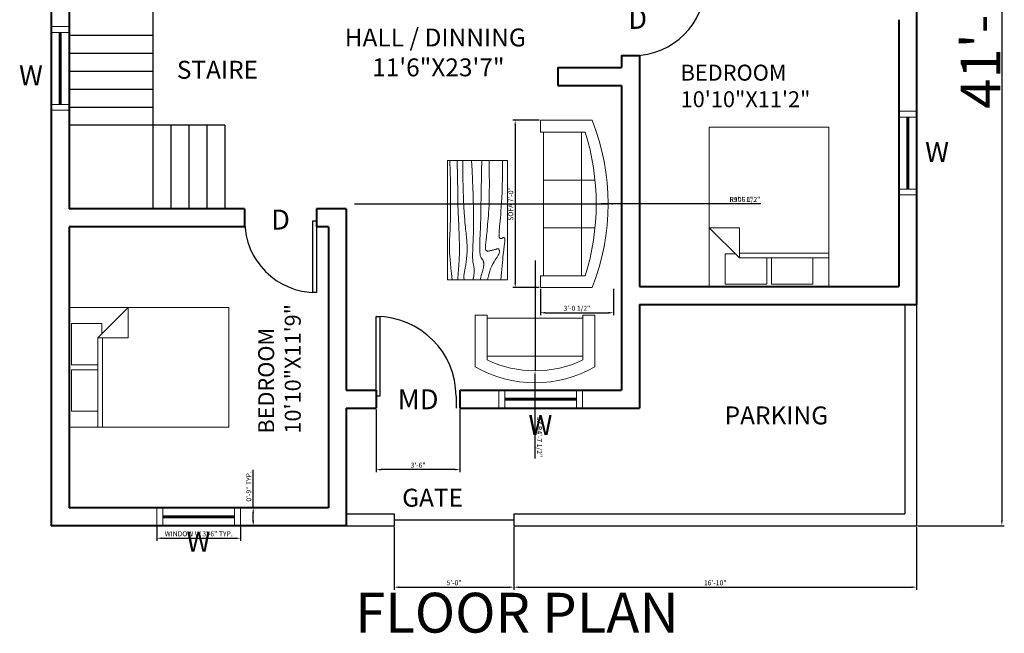
# Model space of a CAD drawing. Units: inches. Extents: x 4878 to 9282, y 5367 to 6617.
# Tile 10 of 14: x 8028 to 8522, y 6010 to 6318. Entities that reach past the tile are written whole.
import ezdxf

# ---------------------------------------------------------------- set-up
doc = ezdxf.new("R2010")
doc.units = ezdxf.units.IN
for name, color, linetype, lineweight in [('A-ANNO-DIMS', 2, 'Continuous', 18), ('A-ANNO-TEXT', 7, 'Continuous', 18), ('A-ANNO-TITL', 3, 'Continuous', 30), ('A-AREA-IDEN', 4, 'Continuous', 18), ('A-DOOR', 3, 'Continuous', 25), ('A-FLOR-STRS', 7, 'Continuous', 25), ('A-FURN', 8, 'Continuous', 18), ('A-GLAZ', 30, 'Continuous', 20), ('A-SITE', 7, 'Continuous', 25), ('A-WALL', 7, 'Continuous', 40)]:
    doc.layers.add(name, color=color, linetype=linetype, lineweight=lineweight)
doc.styles.get("Standard").update_dxf_attribs({"font": 'arial.ttf'})
doc.dimstyles.new('ISO-25', dxfattribs={"dimtxt": 2.5, "dimasz": 2.5, "dimexe": 1.25, "dimexo": 0.625, "dimtad": 1, "dimdec": 0, "dimlunit": 3, "dimtxsty": 'Standard', "dimcen": 2.5, "dimadec": 0, "dimazin": 0, "dimtfac": 1, "dimtdec": 0, "dimtmove": 0, "dimatfit": 3, "dimfxl": 1, "dimarcsym": 0})

# ---------------------------------------------------------------- blocks, each defined once
blk = doc.blocks.new('Bed - Queen')
for p, q in [((0, -80.00003), (0, 0)), ((0, 0), (59.99999, 0)), ((59.99999, 0), (59.99999, -80.00003)), ((7.99999, -1.2), (28.79998, -1.2)), ((7.99999, -14.4), (7.99999, -1.2)), ((28.79998, -1.2), (28.79998, -14.4)), ((31.19999, -1.2), (51.99999, -1.2)), ((31.19999, -14.4), (31.19999, -1.2)), ((51.99999, -1.2), (51.99999, -16.4)), ((0, -14.4), (44.8, -14.4)), ((59.99999, -29.6), (44.8, -14.4)), ((44.8, -14.4), (44.8, -29.6)), ((44.8, -16.8), (0, -16.8)), ((51.99999, -16.4), (46.79936, -16.4)), ((44.8, -29.6), (59.99999, -29.6)), ((59.99999, -80.00003), (0, -80.00003))]:
    blk.add_line(p, q)
blk = doc.blocks.new('Sofa - Roundback 7 ft.')
for p, q in [((-12.00002, -32.4421), (-12.00003, -6.5971)), ((11.99997, -32.4421), (11.99998, -6.5971)), ((-36.000027, -34), (-36.000027, -11.4696)), ((-35.999844, -13.3819), (35.9998, -13.3819)), ((35.99998, -34), (35.99998, -11.4696)), ((-36.000027, -32.4421), (35.99998, -32.4421))]:
    blk.add_line(p, q)
for points in [[(-36.000027, -34), (-42.000027, -34), (-42.000027, -8)], [(41.99998, -8), (41.99998, -34), (35.99998, -34)]]:
    blk.add_lwpolyline(points)
for centre, radius, start, end in [((0, -114.25), 114.25, 68.43141, 111.5686), ((-0.00001, -127.1968), 121.1968, 72.72033, 107.2797)]:
    blk.add_arc(centre, radius, start, end)
blk = doc.blocks.new('Sofa - Roundback Loveseat 5 ft.')
for p, q in [((0, -32.44198), (0, -5.99998)), ((-24, -33.99998), (-24, -11.46958)), ((-23.9998, -13.38178), (23.99986, -13.38178)), ((24.00004, -33.99998), (24.00004, -11.46958)), ((-24, -32.44198), (24.00004, -32.44198))]:
    blk.add_line(p, q)
for points in [[(-24, -33.99998), (-30, -33.99998), (-30, -7.99998)], [(30.00004, -7.99998), (30.00004, -33.99998), (24.00004, -33.99998)]]:
    blk.add_lwpolyline(points)
for centre, radius, start, end in [((0, -60.24998), 60.24998, 60.13715, 119.8628), ((0, -61.38438), 55.38444, 64.32083, 115.6792)]:
    blk.add_arc(centre, radius, start, end)
blk = doc.blocks.new('Table - Rectangular Woodgrain 60 x 30 in.')
for p, q in [((0, 0), (0, -30)), ((60, 0), (0, 0)), ((60, -30), (60, 0)), ((0, -30), (60, -30))]:
    blk.add_line(p, q)
for points in [[(0, -2.4), (4.8155, -2.418), (9.0302, -2.4688), (12.709, -2.5477), (15.9167, -2.65), (18.7181, -2.7711), (21.1781, -2.9063), (23.3616, -3.0508), (25.3333, -3.2), (27.1477, -3.3495), (28.8172, -3.4958), (30.3437, -3.636), (31.7291, -3.7667), (32.9756, -3.8849), (34.0849, -3.9875), (35.059, -4.0714), (35.9, -4.1334), (36.6114, -4.1711), (37.2041, -4.1854), (37.6906, -4.1779), (38.0833, -4.15), (38.3948, -4.1034), (38.6375, -4.0396), (38.8239, -3.9602), (38.9666, -3.8667), (39.0764, -3.7608), (39.1573, -3.6448), (39.2116, -3.521), (39.2416, -3.3917), (39.2498, -3.2593), (39.2385, -3.1261), (39.21, -2.9944), (39.1666, -2.8667), (39.111, -2.7447), (39.0468, -2.6281), (38.978, -2.5163), (38.9083, -2.4083), (38.8418, -2.3035), (38.7823, -2.201), (38.7337, -2.1001), (38.7, -2), (38.6844, -1.9003), (38.6875, -1.8021), (38.7094, -1.707), (38.75, -1.6167), (38.8094, -1.5326), (38.8875, -1.4563), (38.9844, -1.3893), (39.1, -1.3333), (39.2351, -1.2896), (39.3937, -1.2583), (39.5804, -1.2396), (39.8, -1.2333), (40.057, -1.2396), (40.3562, -1.2583), (40.7023, -1.2896), (41.1, -1.3333), (41.5547, -1.3895), (42.0755, -1.4573), (42.6721, -1.5361), (43.3542, -1.625), (44.1316, -1.7233), (45.014, -1.8302), (46.0114, -1.9449), (47.1333, -2.0667), (48.3862, -2.1947), (49.7625, -2.3281), (51.2513, -2.4663), (52.8416, -2.6083), (54.5226, -2.7535), (56.2833, -2.9011), (58.1127, -3.0501), (60, -3.2)], [(0, -9.2), (6.5759, -9.0858), (11.9385, -9.0365), (16.2527, -9.0418), (19.6833, -9.0917), (22.3952, -9.1759), (24.5531, -9.2844), (26.322, -9.4069), (27.8666, -9.5333), (29.3241, -9.6553), (30.7203, -9.7719), (32.0532, -9.8837), (33.3208, -9.9917), (34.5213, -10.0965), (35.6526, -10.199), (36.7128, -10.2999), (37.7, -10.4), (38.6129, -10.4996), (39.4531, -10.5969), (40.223, -10.6895), (40.925, -10.775), (41.5613, -10.8512), (42.1344, -10.9156), (42.6465, -10.966), (43.1, -11), (43.4976, -11.0158), (43.8437, -11.0136), (44.143, -10.9942), (44.4, -10.9583), (44.6195, -10.9069), (44.8062, -10.8406), (44.9648, -10.7603), (45.1, -10.6667), (45.2155, -10.5598), (45.3114, -10.4365), (45.3871, -10.2929), (45.4416, -10.125), (45.4743, -9.929), (45.4844, -9.7011), (45.4709, -9.4371), (45.4333, -9.1333), (45.3716, -8.7883), (45.2896, -8.4104), (45.1919, -8.0107), (45.0833, -7.6), (44.9685, -7.1893), (44.8521, -6.7896), (44.7388, -6.4117), (44.6333, -6.0667), (44.54, -5.7628), (44.4614, -5.4979), (44.4001, -5.2675), (44.3583, -5.0667), (44.3384, -4.8909), (44.3427, -4.7354), (44.3736, -4.5956), (44.4333, -4.4667), (44.5236, -4.3453), (44.6427, -4.2333), (44.7884, -4.1339), (44.9583, -4.05), (45.1501, -3.9849), (45.3614, -3.9417), (45.59, -3.9234), (45.8333, -3.9333), (46.0915, -3.9749), (46.3734, -4.0531), (46.6906, -4.1736), (47.0542, -4.3417), (47.4756, -4.5629), (47.9661, -4.8427), (48.5372, -5.1866), (49.2, -5.6), (49.9676, -6.0844), (50.8594, -6.625), (51.8965, -7.2031), (53.1, -7.8), (54.491, -8.3969), (56.0906, -8.975), (57.9199, -9.5156), (60, -10)], [(0, -12.8), (5.1847, -12.9322), (9.6213, -13.0323), (13.3963, -13.1059), (16.5958, -13.1583), (19.3063, -13.1952), (21.614, -13.2219), (23.6054, -13.2439), (25.3666, -13.2667), (26.9728, -13.2947), (28.4531, -13.3281), (29.8256, -13.3663), (31.1083, -13.4083), (32.3191, -13.4535), (33.476, -13.501), (34.597, -13.5501), (35.7, -13.6), (36.7984, -13.6497), (37.8875, -13.6979), (38.9578, -13.743), (40, -13.7833), (41.0047, -13.8174), (41.9625, -13.8438), (42.864, -13.8607), (43.7, -13.8667), (44.4631, -13.8604), (45.1552, -13.8417), (45.7801, -13.8104), (46.3416, -13.7667), (46.8439, -13.7104), (47.2906, -13.6417), (47.6858, -13.5604), (48.0333, -13.4667), (48.3375, -13.3608), (48.6042, -13.2448), (48.8396, -13.121), (49.05, -12.9917), (49.2417, -12.8593), (49.4208, -12.7261), (49.5937, -12.5944), (49.7667, -12.4667), (49.9452, -12.3451), (50.1323, -12.2313), (50.3303, -12.1268), (50.5416, -12.0333), (50.7686, -11.9524), (51.0135, -11.8854), (51.2788, -11.8341), (51.5666, -11.8), (51.8785, -11.7843), (52.2116, -11.7865), (52.562, -11.8059), (52.926, -11.8417), (53.2998, -11.8931), (53.6795, -11.9594), (54.0614, -12.0397), (54.4416, -12.1333), (54.8223, -12.2401), (55.2293, -12.3625), (55.6942, -12.5037), (56.2489, -12.6667), (56.9251, -12.8547), (57.7545, -13.0708), (58.7689, -13.3182), (60, -13.6)], [(0, -18), (5.124, -17.7273), (9.6609, -17.5057), (13.6705, -17.3303), (17.2125, -17.1958), (20.3467, -17.0973), (23.1328, -17.0297), (25.6307, -16.9878), (27.9, -16.9667), (29.9928, -16.9617), (31.9302, -16.9703), (33.7254, -16.9907), (35.3917, -17.0208), (36.9423, -17.0588), (38.3906, -17.1026), (39.7499, -17.1503), (41.0333, -17.2), (42.2519, -17.2496), (43.4073, -17.2969), (44.4986, -17.3395), (45.525, -17.375), (46.4858, -17.4012), (47.3802, -17.4156), (48.2074, -17.416), (48.9667, -17.4), (49.6583, -17.3662), (50.2872, -17.3167), (50.8595, -17.2547), (51.3812, -17.1833), (51.8584, -17.1057), (52.2971, -17.025), (52.7034, -16.9443), (53.0833, -16.8667), (53.443, -16.7951), (53.789, -16.7313), (54.128, -16.6768), (54.4666, -16.6334), (54.8115, -16.6024), (55.1693, -16.5854), (55.5465, -16.5841), (55.95, -16.6), (56.3828, -16.6337), (56.8346, -16.6823), (57.2915, -16.7418), (57.7396, -16.8084), (58.165, -16.878), (58.5539, -16.9469), (58.8924, -17.0111), (59.1666, -17.0667), (59.3679, -17.1107), (59.5078, -17.1438), (59.6032, -17.1675), (59.6708, -17.1833), (59.7275, -17.193), (59.7901, -17.1979), (59.8753, -17.1998), (60, -17.2)], [(0, -22.4), (8.0098, -22.2501), (14.4094, -22.1011), (19.4168, -21.9535), (23.25, -21.8083), (26.1269, -21.6663), (28.2656, -21.5281), (29.884, -21.3947), (31.2, -21.2667), (32.3967, -21.1448), (33.5172, -21.0292), (34.5697, -20.9198), (35.5625, -20.8167), (36.5037, -20.7198), (37.4015, -20.6292), (38.2642, -20.5448), (39.1, -20.4667), (39.9164, -20.3951), (40.7187, -20.3313), (41.5117, -20.2768), (42.3, -20.2333), (43.0883, -20.2024), (43.8812, -20.1854), (44.6836, -20.1841), (45.5, -20.2), (46.3328, -20.234), (47.1747, -20.2844), (48.0163, -20.3488), (48.8479, -20.425), (49.66, -20.5106), (50.4429, -20.6031), (51.1872, -20.7004), (51.8833, -20.8), (52.5246, -20.8999), (53.1166, -20.9995), (53.6681, -21.0983), (54.1875, -21.1958), (54.6834, -21.2919), (55.1646, -21.3859), (55.6394, -21.4777), (56.1167, -21.5667), (56.6028, -21.6515), (57.0961, -21.7266), (57.5929, -21.7852), (58.0896, -21.8208), (58.5823, -21.8268), (59.0674, -21.7964), (59.5412, -21.723), (60, -21.6)], [(0, -25.2), (8.6355, -25.0504), (15.7026, -24.9031), (21.4049, -24.7606), (25.9458, -24.625), (29.529, -24.4988), (32.3578, -24.3844), (34.6359, -24.284), (36.5667, -24.2), (38.3213, -24.1341), (39.9417, -24.0854), (41.437, -24.0523), (42.8167, -24.0333), (44.0901, -24.0268), (45.2667, -24.0313), (46.3557, -24.0451), (47.3667, -24.0667), (48.309, -24.0947), (49.1928, -24.1287), (50.0284, -24.168), (50.826, -24.2125), (51.5959, -24.2617), (52.3483, -24.3151), (53.0935, -24.3725), (53.8417, -24.4334), (54.6009, -24.497), (55.3699, -24.561), (56.1454, -24.6226), (56.9239, -24.6792), (57.7021, -24.7279), (58.4764, -24.7662), (59.2435, -24.7911), (60, -24.8)], [(0, -28.8), (5.6867, -28.6681), (10.45, -28.5698), (14.407, -28.5012), (17.675, -28.4584), (20.3711, -28.4374), (22.6125, -28.4344), (24.5164, -28.4455), (26.2, -28.4667), (27.762, -28.4947), (29.2276, -28.5281), (30.6033, -28.5663), (31.8958, -28.6084), (33.1118, -28.6535), (34.2578, -28.7011), (35.3405, -28.7501), (36.3666, -28.8), (37.3443, -28.8497), (38.288, -28.8974), (39.2137, -28.9412), (40.1375, -28.9792), (41.0753, -29.0093), (42.0432, -29.0297), (43.0572, -29.0384), (44.1333, -29.0333), (45.2936, -29.0114), (46.5843, -28.9641), (48.0579, -28.8816), (49.7666, -28.7542), (51.7629, -28.5721), (54.0989, -28.3255), (56.8272, -28.0048), (60, -27.6)]]:
    blk.add_lwpolyline(points)
blk = doc.blocks.new('*U18')
for p, q in [((0, 0), (0, -6)), ((40, 0), (40, -6))]:
    blk.add_line(p, q)
blk.add_lwpolyline([(0, 0), (0, 40), (1.75, 40), (1.75, 0)], close=True)
blk.add_arc((0, 0), 40, 0, 90)
blk = doc.blocks.new('*U20')
for p, q in [((-36, 0), (-36, 6)), ((0, 0), (0, 6))]:
    blk.add_line(p, q)
blk.add_lwpolyline([(0, 0), (0, -36), (-1.75, -36), (-1.75, 0)], close=True)
blk.add_arc((0, 0), 36, 180, 270)
blk = doc.blocks.new('*D26')
at = {"layer": 'A-ANNO-DIMS', "color": 0, "lineweight": -2, "transparency": 16777216}
for p, q in [((8478.72, 6557.77), (8522.05, 6557.77)), ((8520.8, 6555.27), (8520.8, 6066.27)), ((8478.72, 6063.77), (8522.05, 6063.77))]:
    blk.add_line(p, q, dxfattribs=at)
at = {"layer": 'A-ANNO-DIMS', "color": 0, "transparency": 16777216}
for points in [[(8520.39, 6555.27), (8521.22, 6555.27), (8520.8, 6557.77)], [(8520.39, 6066.27), (8521.22, 6066.27), (8520.8, 6063.77)]]:
    blk.add_solid(points, dxfattribs=at)
at = {"layer": 'Defpoints', "color": 0, "transparency": 16777216}
for p in [(8478.1, 6557.77), (8478.1, 6063.77), (8520.8, 6063.77)]:
    blk.add_point(p, dxfattribs=at)
at = {"layer": 'A-ANNO-DIMS', "color": 0, "transparency": 16777216, "insert": (8510.14, 6310.77), "char_height": 2.5, "attachment_point": 5, "rotation": 90}
blk.add_mtext('{\\H8x;41\'-2"}', dxfattribs=at)
blk = doc.blocks.new('WINDOW-PLAN-36IN')
for p, q in [((0, 0), (0, 9)), ((3, 0), (3, 9)), ((3, 5), (39, 5)), ((39, 0), (39, 9)), ((42, 0), (42, 9)), ((3, 4.5), (39, 4.5)), ((3, 4), (39, 4))]:
    blk.add_line(p, q)
blk = doc.blocks.new('*D39')
at = {"layer": 'A-ANNO-DIMS', "color": 0, "lineweight": -2, "transparency": 16777216}
for p, q in [((8097.1, 6063.15), (8097.1, 6056.22)), ((8139.1, 6063.15), (8139.1, 6056.22)), ((8099.6, 6057.47), (8136.6, 6057.47))]:
    blk.add_line(p, q, dxfattribs=at)
at = {"layer": 'A-ANNO-DIMS', "color": 0, "transparency": 16777216}
for points in [[(8099.6, 6057.89), (8099.6, 6057.05), (8097.1, 6057.47)], [(8136.6, 6057.89), (8136.6, 6057.05), (8139.1, 6057.47)]]:
    blk.add_solid(points, dxfattribs=at)
at = {"layer": 'Defpoints', "color": 0, "transparency": 16777216}
for p in [(8097.1, 6063.77), (8139.1, 6063.77), (8139.1, 6057.47)]:
    blk.add_point(p, dxfattribs=at)
at = {"layer": 'A-ANNO-DIMS', "color": 0, "transparency": 16777216, "insert": (8118.1, 6059.39), "char_height": 2.5, "attachment_point": 5}
blk.add_mtext('WINDOW W 3\'-6" TYP.', dxfattribs=at)
blk = doc.blocks.new('*D40')
at = {"layer": 'A-ANNO-DIMS', "color": 0, "lineweight": -2, "transparency": 16777216}
for p, q in [((8145.4, 6072.77), (8145.4, 6091.76)), ((8139.72, 6072.77), (8146.65, 6072.77)), ((8145.4, 6066.27), (8145.4, 6070.27)), ((8139.72, 6063.77), (8146.65, 6063.77))]:
    blk.add_line(p, q, dxfattribs=at)
at = {"layer": 'A-ANNO-DIMS', "color": 0, "transparency": 16777216}
for points in [[(8144.98, 6070.27), (8145.81, 6070.27), (8145.4, 6072.77)], [(8144.98, 6066.27), (8145.81, 6066.27), (8145.4, 6063.77)]]:
    blk.add_solid(points, dxfattribs=at)
at = {"layer": 'Defpoints', "color": 0, "transparency": 16777216}
for p in [(8139.1, 6072.77), (8145.4, 6072.77), (8139.1, 6063.77)]:
    blk.add_point(p, dxfattribs=at)
at = {"layer": 'A-ANNO-DIMS', "color": 0, "transparency": 16777216, "insert": (8143.49, 6083.52), "char_height": 2.5, "attachment_point": 5, "rotation": 90}
blk.add_mtext('0\'-9" TYP.', dxfattribs=at)
blk = doc.blocks.new('*D63')
at = {"layer": 'A-ANNO-DIMS', "color": 0, "lineweight": -2, "transparency": 16777216}
for p, q in [((8288.76, 6267.27), (8275.54, 6267.27)), ((8276.79, 6264.77), (8276.79, 6185.77)), ((8288.76, 6183.27), (8275.54, 6183.27))]:
    blk.add_line(p, q, dxfattribs=at)
at = {"layer": 'A-ANNO-DIMS', "color": 0, "transparency": 16777216}
for points in [[(8276.37, 6264.77), (8277.21, 6264.77), (8276.79, 6267.27)], [(8276.37, 6185.77), (8277.21, 6185.77), (8276.79, 6183.27)]]:
    blk.add_solid(points, dxfattribs=at)
at = {"layer": 'Defpoints', "color": 0, "transparency": 16777216}
for p in [(8289.39, 6267.27), (8276.79, 6183.27), (8289.39, 6183.27)]:
    blk.add_point(p, dxfattribs=at)
at = {"layer": 'A-ANNO-DIMS', "color": 0, "transparency": 16777216, "insert": (8274.87, 6225.27), "char_height": 2.5, "attachment_point": 5, "rotation": 90}
blk.add_mtext('SOFA 7\'-0"', dxfattribs=at)
blk = doc.blocks.new('*D64')
at = {"layer": 'A-ANNO-DIMS', "color": 0, "lineweight": -2, "transparency": 16777216}
for p, q in [((8289.39, 6182.64), (8289.39, 6169.42)), ((8326.06, 6182.64), (8326.06, 6169.42)), ((8291.89, 6170.67), (8323.56, 6170.67))]:
    blk.add_line(p, q, dxfattribs=at)
at = {"layer": 'A-ANNO-DIMS', "color": 0, "transparency": 16777216}
for points in [[(8291.89, 6171.08), (8291.89, 6170.25), (8289.39, 6170.67)], [(8323.56, 6171.08), (8323.56, 6170.25), (8326.06, 6170.67)]]:
    blk.add_solid(points, dxfattribs=at)
at = {"layer": 'Defpoints', "color": 0, "transparency": 16777216}
for p in [(8289.39, 6183.27), (8326.06, 6183.27), (8326.06, 6170.67)]:
    blk.add_point(p, dxfattribs=at)
at = {"layer": 'A-ANNO-DIMS', "color": 0, "transparency": 16777216, "insert": (8307.72, 6172.58), "char_height": 2.5, "attachment_point": 5}
blk.add_mtext('3\'-0 1/2"', dxfattribs=at)
blk = doc.blocks.new('*D109')
at = {"layer": 'A-ANNO-DIMS', "color": 0, "lineweight": -2, "transparency": 16777216}
for p, q in [((8207.1, 6122.15), (8207.1, 6090.67)), ((8249.1, 6122.15), (8249.1, 6090.67)), ((8246.6, 6091.92), (8209.6, 6091.92))]:
    blk.add_line(p, q, dxfattribs=at)
at = {"layer": 'A-ANNO-DIMS', "color": 0, "transparency": 16777216}
for points in [[(8209.6, 6092.34), (8209.6, 6091.5), (8207.1, 6091.92)], [(8246.6, 6092.34), (8246.6, 6091.5), (8249.1, 6091.92)]]:
    blk.add_solid(points, dxfattribs=at)
at = {"layer": 'Defpoints', "color": 0, "transparency": 16777216}
for p in [(8207.1, 6122.77), (8249.1, 6122.77), (8207.1, 6091.92)]:
    blk.add_point(p, dxfattribs=at)
at = {"layer": 'A-ANNO-DIMS', "color": 0, "transparency": 16777216, "insert": (8228.1, 6093.82), "char_height": 2.5, "attachment_point": 5}
blk.add_mtext('3\'-6"', dxfattribs=at)
blk = doc.blocks.new('*D111')
at = {"layer": 'A-ANNO-DIMS', "color": 0, "lineweight": -2, "transparency": 16777216}
for p, q in [((8216.1, 6063.15), (8216.1, 6031.67)), ((8276.1, 6063.15), (8276.1, 6031.67)), ((8218.6, 6032.92), (8273.6, 6032.92))]:
    blk.add_line(p, q, dxfattribs=at)
at = {"layer": 'A-ANNO-DIMS', "color": 0, "transparency": 16777216}
for points in [[(8218.6, 6033.34), (8218.6, 6032.5), (8216.1, 6032.92)], [(8273.6, 6033.34), (8273.6, 6032.5), (8276.1, 6032.92)]]:
    blk.add_solid(points, dxfattribs=at)
at = {"layer": 'Defpoints', "color": 0, "transparency": 16777216}
for p in [(8216.1, 6063.77), (8276.1, 6063.77), (8276.1, 6032.92)]:
    blk.add_point(p, dxfattribs=at)
at = {"layer": 'A-ANNO-DIMS', "color": 0, "transparency": 16777216, "insert": (8246.1, 6034.82), "char_height": 2.5, "attachment_point": 5}
blk.add_mtext('5\'-0"', dxfattribs=at)
blk = doc.blocks.new('*D112')
at = {"layer": 'A-ANNO-DIMS', "color": 0, "lineweight": -2, "transparency": 16777216}
for p, q in [((8276.1, 6063.15), (8276.1, 6031.67)), ((8478.1, 6063.15), (8478.1, 6031.67)), ((8278.6, 6032.92), (8475.6, 6032.92))]:
    blk.add_line(p, q, dxfattribs=at)
at = {"layer": 'A-ANNO-DIMS', "color": 0, "transparency": 16777216}
for points in [[(8278.6, 6033.34), (8278.6, 6032.5), (8276.1, 6032.92)], [(8475.6, 6033.34), (8475.6, 6032.5), (8478.1, 6032.92)]]:
    blk.add_solid(points, dxfattribs=at)
at = {"layer": 'Defpoints', "color": 0, "transparency": 16777216}
for p in [(8276.1, 6063.77), (8478.1, 6063.77), (8478.1, 6032.92)]:
    blk.add_point(p, dxfattribs=at)
at = {"layer": 'A-ANNO-DIMS', "color": 0, "transparency": 16777216, "insert": (8377.1, 6034.82), "char_height": 2.5, "attachment_point": 5}
blk.add_mtext('16\'-10"', dxfattribs=at)
blk = doc.blocks.new('*D123')
at = {"layer": 'A-ANNO-DIMS', "color": 0, "lineweight": -2, "transparency": 16777216}
for p, q in [((8286.73, 6196.91), (8286.73, 6141.53)), ((8286.73, 6097.55), (8286.73, 6139.03))]:
    blk.add_line(p, q, dxfattribs=at)
at = {"layer": 'A-ANNO-DIMS', "color": 0, "transparency": 16777216}
blk.add_solid([(8287.15, 6139.03), (8286.32, 6139.03), (8286.73, 6141.53)], dxfattribs=at)
at = {"layer": 'Defpoints', "color": 0, "transparency": 16777216}
for p in [(8286.73, 6196.91), (8286.73, 6141.53)]:
    blk.add_point(p, dxfattribs=at)
at = {"layer": 'A-ANNO-DIMS', "color": 0, "transparency": 16777216, "insert": (8288.65, 6108.29), "char_height": 2.5, "attachment_point": 5, "rotation": 270.0004}
blk.add_mtext('3X R4\'-7 1/2"', dxfattribs=at)
blk = doc.blocks.new('*D124')
at = {"layer": 'A-ANNO-DIMS', "color": 0, "lineweight": -2, "transparency": 16777216}
for p, q in [((8196.19, 6225.27), (8317.39, 6225.27)), ((8396.22, 6225.27), (8319.89, 6225.27))]:
    blk.add_line(p, q, dxfattribs=at)
at = {"layer": 'A-ANNO-DIMS', "color": 0, "transparency": 16777216}
blk.add_solid([(8319.89, 6225.68), (8319.89, 6224.85), (8317.39, 6225.27)], dxfattribs=at)
at = {"layer": 'Defpoints', "color": 0, "transparency": 16777216}
for p in [(8196.19, 6225.27), (8317.39, 6225.27)]:
    blk.add_point(p, dxfattribs=at)
at = {"layer": 'A-ANNO-DIMS', "color": 0, "transparency": 16777216, "insert": (8390.11, 6227.17), "char_height": 2.5, "attachment_point": 5, "rotation": 360}
blk.add_mtext('R10\'-1"', dxfattribs=at)
blk = doc.blocks.new('*D125')
at = {"layer": 'A-ANNO-DIMS', "color": 0, "lineweight": -2, "transparency": 16777216}
for p, q in [((8209.14, 6225.27), (8323.39, 6225.27)), ((8400, 6225.27), (8325.89, 6225.27))]:
    blk.add_line(p, q, dxfattribs=at)
at = {"layer": 'A-ANNO-DIMS', "color": 0, "transparency": 16777216}
blk.add_solid([(8325.89, 6225.68), (8325.89, 6224.85), (8323.39, 6225.27)], dxfattribs=at)
at = {"layer": 'Defpoints', "color": 0, "transparency": 16777216}
for p in [(8209.14, 6225.27), (8323.39, 6225.27)]:
    blk.add_point(p, dxfattribs=at)
at = {"layer": 'A-ANNO-DIMS', "color": 0, "transparency": 16777216, "insert": (8391.94, 6227.18), "char_height": 2.5, "attachment_point": 5, "rotation": 360}
blk.add_mtext('R9\'-6 1/2"', dxfattribs=at)

msp = doc.modelspace()

# ---------------------------------------------------------------- linework, layer by layer
at = {"layer": 'A-FLOR-STRS'}
for p, q in [((8095.1, 6363.77), (8095.1, 6222.77)), ((8095.1, 6309.77), (8053.1, 6309.77)), ((8095.1, 6300.77), (8053.1, 6300.77)), ((8095.1, 6291.77), (8053.1, 6291.77)), ((8095.1, 6291.77), (8053.1, 6291.77)), ((8095.1, 6282.77), (8053.1, 6282.77)), ((8095.1, 6273.77), (8053.1, 6273.77)), ((8131.1, 6264.77), (8053.1, 6264.77)), ((8104.1, 6264.77), (8104.1, 6222.77)), ((8113.1, 6264.77), (8113.1, 6222.77)), ((8122.1, 6264.77), (8122.1, 6222.77)), ((8131.1, 6264.77), (8131.1, 6222.77))]:
    msp.add_line(p, q, dxfattribs=at)
at = {"layer": 'A-SITE'}
for p, q in [((8472.1, 6174.77), (8472.1, 6069.77)), ((8478.1, 6174.77), (8478.1, 6063.77)), ((8192.1, 6069.77), (8216.1, 6069.77)), ((8216.1, 6069.77), (8216.1, 6063.77)), ((8276.1, 6069.77), (8276.1, 6063.77)), ((8276.1, 6069.77), (8472.1, 6069.77)), ((8192.1, 6063.77), (8216.1, 6063.77)), ((8216.1, 6066.77), (8276.1, 6066.77)), ((8276.1, 6063.77), (8478.1, 6063.77))]:
    msp.add_line(p, q, dxfattribs=at)
at = {"layer": 'A-WALL'}
for p, q in [((8478.1, 6557.77), (8478.1, 6174.77)), ((8044.1, 6363.77), (8044.1, 6063.77)), ((8053.1, 6363.77), (8053.1, 6222.77)), ((8469.1, 6317.77), (8469.1, 6183.77)), ((8330.1, 6299.77), (8330.1, 6293.77)), ((8330.1, 6299.77), (8339.1, 6299.77)), ((8330.1, 6299.77), (8330.1, 6293.77)), ((8339.1, 6299.77), (8339.1, 6183.77)), ((8298.1, 6293.77), (8330.1, 6293.77)), ((8298.1, 6293.77), (8298.1, 6284.77)), ((8298.1, 6284.77), (8330.1, 6284.77)), ((8330.1, 6284.77), (8330.1, 6131.77)), ((8141.1, 6222.77), (8053.1, 6222.77)), ((8141.1, 6222.77), (8141.1, 6213.77)), ((8192.1, 6222.77), (8177.1, 6222.77)), ((8177.1, 6222.77), (8177.1, 6213.77)), ((8192.1, 6222.77), (8192.1, 6131.77)), ((8141.1, 6213.77), (8053.1, 6213.77)), ((8053.1, 6213.77), (8053.1, 6072.77)), ((8183.1, 6213.77), (8177.1, 6213.77)), ((8183.1, 6213.77), (8183.1, 6072.77)), ((8339.1, 6183.77), (8469.1, 6183.77)), ((8339.1, 6174.77), (8478.1, 6174.77)), ((8339.1, 6174.77), (8339.1, 6122.77)), ((8192.1, 6131.77), (8207.1, 6131.77)), ((8207.1, 6131.77), (8207.1, 6122.77)), ((8249.1, 6131.77), (8330.1, 6131.77)), ((8249.1, 6131.77), (8249.1, 6122.77)), ((8192.1, 6122.77), (8207.1, 6122.77)), ((8192.1, 6122.77), (8192.1, 6063.77)), ((8249.1, 6122.77), (8339.1, 6122.77)), ((8183.1, 6072.77), (8053.1, 6072.77)), ((8192.1, 6063.77), (8044.1, 6063.77))]:
    msp.add_line(p, q, dxfattribs=at)

# ---------------------------------------------------------------- block references
at = {"layer": 'A-DOOR', "rotation": 90}
msp.add_blockref('*U20', (8336.1, 6335.77), dxfattribs=at)
at = {"layer": 'A-DOOR'}
for name, p in [('*U20', (8177.1, 6216.77)), ('*U18', (8207.1, 6128.77))]:
    msp.add_blockref(name, p, dxfattribs=at)
at = {"layer": 'A-FURN'}
for name, p, rotation in [('Sofa - Roundback 7 ft.', (8323.39, 6225.27), 270), ('Bed - Queen', (8434.1, 6183.77), 180), ('Table - Rectangular Woodgrain 60 x 30 in.', (8272.85, 6247.12), 270), ('Bed - Queen', (8053.1, 6113.27), 90), ('Sofa - Roundback Loveseat 5 ft.', (8286.73, 6135.53), 180)]:
    msp.add_blockref(name, p, dxfattribs=dict(at, rotation=rotation))
at = {"layer": 'A-GLAZ', "extrusion": (0, 0, -1), "zscale": -1, "rotation": 90}
for p in [(-8044.1, 6272.27), (-8469.1, 6229.77)]:
    msp.add_blockref('WINDOW-PLAN-36IN', p, dxfattribs=at)
at = {"layer": 'A-GLAZ'}
for p in [(8268.6, 6122.77), (8097.1, 6063.77)]:
    msp.add_blockref('WINDOW-PLAN-36IN', p, dxfattribs=at)

# ---------------------------------------------------------------- texts
at = {"layer": 'A-ANNO-TEXT', "attachment_point": 1}
for s, width, insert, char_height in [('D', 376.4819, (8333.51, 6323.15), 10), ('STAIRE', 360.8658, (8107.09, 6297.13), 9), ('W', 613.0579, (8027.95, 6294.89), 10), ('W', 613.0579, (8482.33, 6256.4), 10), ('D', 376.4819, (8154.42, 6222.41), 10), ('MD', 613.0579, (8217.88, 6132.21), 10), ('W', 613.0579, (8283.44, 6119.28), 10), ('GATE', 360.8658, (8220.1, 6082.33), 9), ('W', 613.0579, (8111.95, 6060.72), 10)]:
    msp.add_mtext_dynamic_manual_height_columns(s, width=width, gutter_width=12.5, heights=[0], dxfattribs=dict(at, insert=insert, char_height=char_height))
at = {"layer": 'A-ANNO-TITL', "insert": (8196.56, 6030.11), "char_height": 20, "attachment_point": 1}
msp.add_mtext_dynamic_manual_height_columns('FLOOR PLAN', width=599.8964, gutter_width=12.5, heights=[0], dxfattribs=at)
at = {"layer": 'A-AREA-IDEN', "attachment_point": 1}
for s, width, insert, char_height in [('HALL / DINNING\\P     11\'6"X23\'7"', 438.0615, (8191.28, 6313.33), 9), ('BEDROOM\\P10\'10"X11\'2"', 304.9234, (8359.74, 6295.18), 8), ('PARKING', 360.8658, (8381.79, 6123.63), 9)]:
    msp.add_mtext_dynamic_manual_height_columns(s, width=width, gutter_width=12.5, heights=[0], dxfattribs=dict(at, insert=insert, char_height=char_height))
at = {"layer": 'A-AREA-IDEN', "insert": (8147.91, 6109.99), "char_height": 8, "attachment_point": 1, "rotation": 90}
msp.add_mtext_dynamic_manual_height_columns('BEDROOM\\P10\'10"X11\'9"', width=304.9234, gutter_width=12.5, heights=[0], dxfattribs=at)

# ---------------------------------------------------------------- dimensions: what is measured, and where the dimension line sits
at = {"layer": 'A-ANNO-DIMS'}
for base, p1, p2, angle, text, override, picture, middle in [((8520.8, 6063.77), (8478.1, 6557.77), (8478.1, 6063.77), 90, '{\\H8x;<>}', {"dimclrd": 0, "dimclre": 0, "dimclrt": 0}, '*D26', (8510.14, 6310.77)), ((8276.79, 6183.27), (8289.39, 6267.27), (8289.39, 6183.27), 270, 'SOFA <>', {"dimdec": 1, "dimlfac": 1, "dimrnd": 0, "dimzin": 1, "dimdsep": 46, "dimlunit": 4, "dimfrac": 2}, '*D63', (8274.87, 6225.27)), ((8145.4, 6072.77), (8139.1, 6063.77), (8139.1, 6072.77), 90, '<> TYP.', {"dimdec": 1, "dimlfac": 1, "dimrnd": 0, "dimzin": 1, "dimdsep": 46, "dimlunit": 4, "dimfrac": 2}, '*D40', (8143.49, 6083.52))]:
    dim = msp.add_linear_dim(base=base, p1=p1, p2=p2, angle=angle, text=text, dimstyle='ISO-25', override=override, dxfattribs=at)
    dim.commit()
    dim.dimension.update_dxf_attribs({"geometry": picture, "text_midpoint": middle})
for center, mpoint, picture, middle in [((8196.19, 6225.27), (8317.39, 6225.27), '*D124', (8390.11, 6225.27)), ((8209.138592, 6225.26601), (8323.388592, 6225.266), '*D125', (8391.938592, 6225.265994))]:
    dim = msp.add_radius_dim(center=center, mpoint=mpoint, dimstyle='ISO-25', override={"dimdec": 1, "dimlfac": 1, "dimrnd": 0, "dimzin": 1, "dimdsep": 46, "dimlunit": 4, "dimfrac": 2}, dxfattribs=at)
    dim.commit()
    dim.dimension.update_dxf_attribs({"geometry": picture, "text_midpoint": middle, "dimtype": 164})
dim = msp.add_radius_dim(center=(8286.73, 6196.91), mpoint=(8286.73, 6141.53), text='3X <>', dimstyle='ISO-25', override={"dimdec": 1, "dimlfac": 1, "dimrnd": 0, "dimzin": 1, "dimdsep": 46, "dimlunit": 4, "dimfrac": 2}, dxfattribs=at)
dim.commit()
dim.dimension.update_dxf_attribs({"geometry": '*D123', "text_midpoint": (8286.73, 6108.29), "dimtype": 164})
for base, p1, p2, picture, middle in [((8326.06, 6170.67), (8289.39, 6183.27), (8326.06, 6183.27), '*D64', (8307.72, 6172.58)), ((8276.1, 6032.92), (8216.1, 6063.77), (8276.1, 6063.77), '*D111', (8246.1, 6034.82)), ((8478.1, 6032.92), (8276.1, 6063.77), (8478.1, 6063.77), '*D112', (8377.1, 6034.82))]:
    dim = msp.add_linear_dim(base=base, p1=p1, p2=p2, dimstyle='ISO-25', override={"dimdec": 1, "dimlfac": 1, "dimrnd": 0, "dimzin": 1, "dimdsep": 46, "dimlunit": 4, "dimfrac": 2}, dxfattribs=at)
    dim.commit()
    dim.dimension.update_dxf_attribs({"geometry": picture, "text_midpoint": middle})
dim = msp.add_linear_dim(base=(8207.1, 6091.92), p1=(8249.1, 6122.77), p2=(8207.1, 6122.77), angle=180, dimstyle='ISO-25', override={"dimdec": 1, "dimlfac": 1, "dimrnd": 0, "dimzin": 1, "dimdsep": 46, "dimlunit": 4, "dimfrac": 2}, dxfattribs=at)
dim.commit()
dim.dimension.update_dxf_attribs({"geometry": '*D109', "text_midpoint": (8228.1, 6093.82)})
dim = msp.add_linear_dim(base=(8139.1, 6057.47), p1=(8097.1, 6063.77), p2=(8139.1, 6063.77), text='WINDOW W <> TYP.', dimstyle='ISO-25', override={"dimdec": 1, "dimlfac": 1, "dimrnd": 0, "dimzin": 1, "dimdsep": 46, "dimlunit": 4, "dimfrac": 2}, dxfattribs=at)
dim.commit()
dim.dimension.update_dxf_attribs({"geometry": '*D39', "text_midpoint": (8118.1, 6059.39)})

doc.saveas('drawing.dxf')
